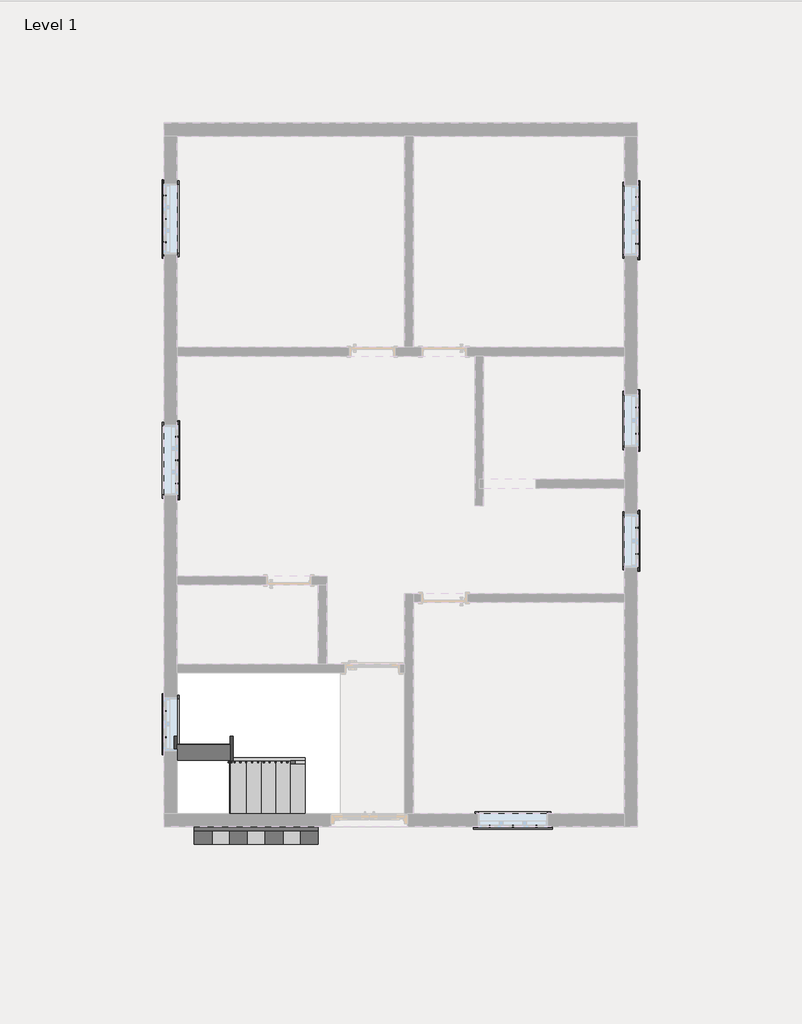
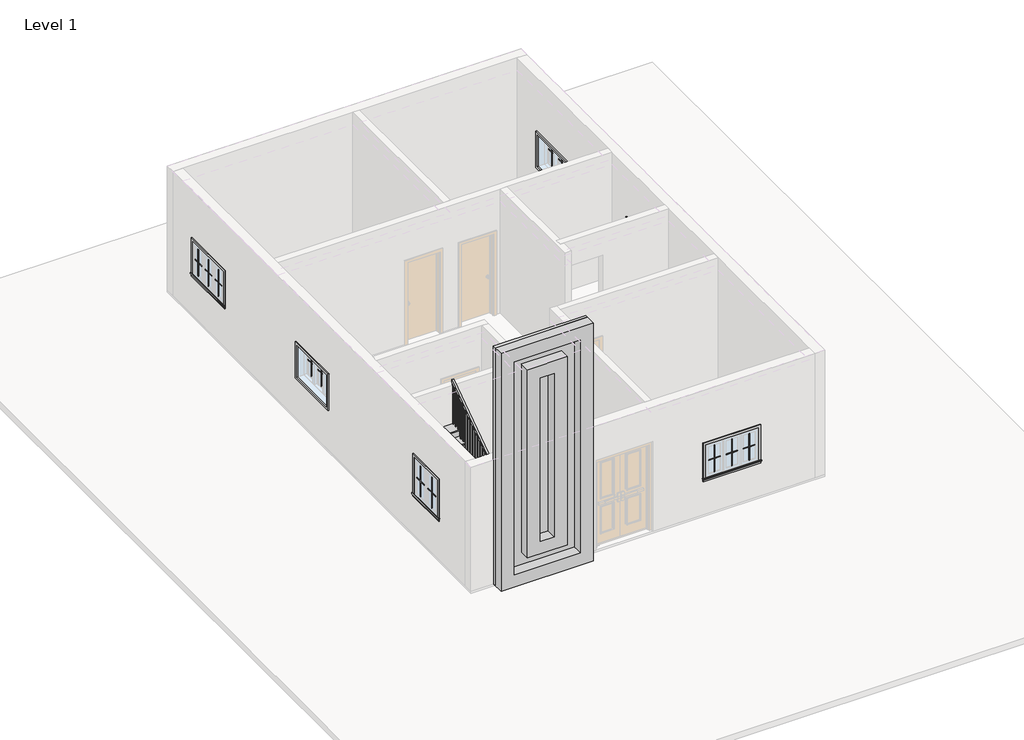
# One storey, part 2 of 2: 33 proxies, 6 members, 2 stair flights, 1 railing.
"""IFC4 building model written with IfcOpenShell, lengths in millimetres."""

from ifc_helpers import new_model, si_unit, frame, origin, place, context, project, spatial, polyline, outline, extrude, faceted_brep, transform, mapped, element, save
from components import design_design_9549e9b3, m_muntin_pattern_2x2_m_muntin_pattern_2x2_777d393c, m_muntin_pattern_2x2_m_muntin_pattern_2x2_fa3d06ac, m_muntin_pattern_2x2_m_muntin_pattern_2x2_55460d9e, m_muntin_pattern_2x2_m_muntin_pattern_2x2_a9b7b7a9, m_trim_window_exterior_flat_with_sill_3a557199, m_trim_window_exterior_flat_with_sill_8fa486dc, m_trim_window_interior_flat_picture_frame_580345df, m_trim_window_interior_flat_picture_frame_b6dd03a6, stair_flight_0f448409, stair_flight_de56df94

model = new_model("IFC4")

# Units and contexts
model_context = context("Model", 3, world=origin())
ifc_project = project(units=[si_unit("LENGTHUNIT", "METRE", prefix="MILLI")], contexts=[model_context])

# Site, building, storey
site = spatial("IfcSite", under=ifc_project)
building = spatial("IfcBuilding", under=site)
storey = spatial("IfcBuildingStorey", under=building, Name="Level 1", Elevation=0.0)

# Proxies
placement = place(None, origin())
design_design_shape = design_design_9549e9b3(model_context)
element("IfcBuildingElementProxy", 1, Name="DESIGN : DESIGN", ObjectType="DESIGN : DESIGN", at=placement, inside=storey, context=model_context, shape_type="MappedRepresentation", body=[
    mapped(design_design_shape, transform((0.0, 0.0, 0.0), x_axis=(1.0, 0.0, 0.0), y_axis=(0.0, 1.0, 0.0), z_axis=(0.0, 0.0, 1.0))),
])
m_muntin_pattern_2x2_m_muntin_pattern_2x2_shape = m_muntin_pattern_2x2_m_muntin_pattern_2x2_777d393c(model_context)
element("IfcBuildingElementProxy", 2, Name="M_Muntin Pattern_2x2 : M_Muntin Pattern_2x2", ObjectType="M_Muntin Pattern_2x2 : M_Muntin Pattern_2x2", at=placement, inside=storey, context=model_context, shape_type="MappedRepresentation", body=[
    mapped(m_muntin_pattern_2x2_m_muntin_pattern_2x2_shape, transform((-5759.4629317, 4113.1478103, 1111.25), x_axis=(0.0, 1.0, 0.0), y_axis=(-1.0, 0.0, 0.0), z_axis=(0.0, 0.0, 1.0))),
])
element("IfcBuildingElementProxy", 3, Name="M_Muntin Pattern_2x2 : M_Muntin Pattern_2x2", ObjectType="M_Muntin Pattern_2x2 : M_Muntin Pattern_2x2", at=placement, inside=storey, context=model_context, shape_type="MappedRepresentation", body=[
    mapped(m_muntin_pattern_2x2_m_muntin_pattern_2x2_shape, transform((2425.6870683, 4896.314477, 969.85), x_axis=(0.0, -1.0, 0.0), y_axis=(1.0, 0.0, 0.0), z_axis=(0.0, 0.0, 1.0))),
])
element("IfcBuildingElementProxy", 4, Name="M_Muntin Pattern_2x2 : M_Muntin Pattern_2x2", ObjectType="M_Muntin Pattern_2x2 : M_Muntin Pattern_2x2", at=placement, inside=storey, context=model_context, shape_type="MappedRepresentation", body=[
    mapped(m_muntin_pattern_2x2_m_muntin_pattern_2x2_shape, transform((-5549.9129317, 743.414477, 1111.25), x_axis=(0.0, -1.0, 0.0), y_axis=(1.0, 0.0, 0.0), z_axis=(0.0, 0.0, 1.0))),
])
element("IfcBuildingElementProxy", 5, Name="M_Muntin Pattern_2x2 : M_Muntin Pattern_2x2", ObjectType="M_Muntin Pattern_2x2 : M_Muntin Pattern_2x2", at=placement, inside=storey, context=model_context, shape_type="MappedRepresentation", body=[
    mapped(m_muntin_pattern_2x2_m_muntin_pattern_2x2_shape, transform((680.4954017, -6001.3438563, 969.85), x_axis=(-1.0, 0.0, 0.0), y_axis=(0.0, -1.0, 0.0), z_axis=(0.0, 0.0, 1.0))),
])
m_muntin_pattern_2x2_m_muntin_pattern_2x2_2_shape = m_muntin_pattern_2x2_m_muntin_pattern_2x2_fa3d06ac(model_context)
element("IfcBuildingElementProxy", 6, Name="M_Muntin Pattern_2x2 : M_Muntin Pattern_2x2", ObjectType="M_Muntin Pattern_2x2 : M_Muntin Pattern_2x2", at=placement, inside=storey, context=model_context, shape_type="MappedRepresentation", body=[
    mapped(m_muntin_pattern_2x2_m_muntin_pattern_2x2_2_shape, transform((-5759.4629317, 4921.714477, 1111.25), x_axis=(0.0, -1.0, 0.0), y_axis=(1.0, 0.0, 0.0), z_axis=(0.0, 0.0, 1.0))),
])
element("IfcBuildingElementProxy", 7, Name="M_Muntin Pattern_2x2 : M_Muntin Pattern_2x2", ObjectType="M_Muntin Pattern_2x2 : M_Muntin Pattern_2x2", at=placement, inside=storey, context=model_context, shape_type="MappedRepresentation", body=[
    mapped(m_muntin_pattern_2x2_m_muntin_pattern_2x2_2_shape, transform((-5759.4629317, 4517.4311437, 1111.25), x_axis=(0.0, -1.0, 0.0), y_axis=(1.0, 0.0, 0.0), z_axis=(0.0, 0.0, 1.0))),
])
element("IfcBuildingElementProxy", 8, Name="M_Muntin Pattern_2x2 : M_Muntin Pattern_2x2", ObjectType="M_Muntin Pattern_2x2 : M_Muntin Pattern_2x2", at=placement, inside=storey, context=model_context, shape_type="MappedRepresentation", body=[
    mapped(m_muntin_pattern_2x2_m_muntin_pattern_2x2_2_shape, transform((2425.6870683, 4087.7478103, 969.85), x_axis=(0.0, 1.0, 0.0), y_axis=(-1.0, 0.0, 0.0), z_axis=(0.0, 0.0, 1.0))),
])
element("IfcBuildingElementProxy", 9, Name="M_Muntin Pattern_2x2 : M_Muntin Pattern_2x2", ObjectType="M_Muntin Pattern_2x2 : M_Muntin Pattern_2x2", at=placement, inside=storey, context=model_context, shape_type="MappedRepresentation", body=[
    mapped(m_muntin_pattern_2x2_m_muntin_pattern_2x2_2_shape, transform((2425.6870683, 4492.0311437, 969.85), x_axis=(0.0, 1.0, 0.0), y_axis=(-1.0, 0.0, 0.0), z_axis=(0.0, 0.0, 1.0))),
])
element("IfcBuildingElementProxy", 10, Name="M_Muntin Pattern_2x2 : M_Muntin Pattern_2x2", ObjectType="M_Muntin Pattern_2x2 : M_Muntin Pattern_2x2", at=placement, inside=storey, context=model_context, shape_type="MappedRepresentation", body=[
    mapped(m_muntin_pattern_2x2_m_muntin_pattern_2x2_2_shape, transform((-5549.9129317, -65.1521897, 1111.25), x_axis=(0.0, 1.0, 0.0), y_axis=(-1.0, 0.0, 0.0), z_axis=(0.0, 0.0, 1.0))),
])
element("IfcBuildingElementProxy", 11, Name="M_Muntin Pattern_2x2 : M_Muntin Pattern_2x2", ObjectType="M_Muntin Pattern_2x2 : M_Muntin Pattern_2x2", at=placement, inside=storey, context=model_context, shape_type="MappedRepresentation", body=[
    mapped(m_muntin_pattern_2x2_m_muntin_pattern_2x2_2_shape, transform((-5549.9129317, 339.1311437, 1111.25), x_axis=(0.0, 1.0, 0.0), y_axis=(-1.0, 0.0, 0.0), z_axis=(0.0, 0.0, 1.0))),
])
element("IfcBuildingElementProxy", 12, Name="M_Muntin Pattern_2x2 : M_Muntin Pattern_2x2", ObjectType="M_Muntin Pattern_2x2 : M_Muntin Pattern_2x2", at=placement, inside=storey, context=model_context, shape_type="MappedRepresentation", body=[
    mapped(m_muntin_pattern_2x2_m_muntin_pattern_2x2_2_shape, transform((-128.071265, -6001.3438563, 969.85), x_axis=(1.0, 0.0, 0.0), y_axis=(0.0, 1.0, 0.0), z_axis=(0.0, 0.0, 1.0))),
])
element("IfcBuildingElementProxy", 13, Name="M_Muntin Pattern_2x2 : M_Muntin Pattern_2x2", ObjectType="M_Muntin Pattern_2x2 : M_Muntin Pattern_2x2", at=placement, inside=storey, context=model_context, shape_type="MappedRepresentation", body=[
    mapped(m_muntin_pattern_2x2_m_muntin_pattern_2x2_2_shape, transform((276.2120683, -6001.3438563, 969.85), x_axis=(1.0, 0.0, 0.0), y_axis=(0.0, 1.0, 0.0), z_axis=(0.0, 0.0, 1.0))),
])
m_muntin_pattern_2x2_m_muntin_pattern_2x2_3_shape = m_muntin_pattern_2x2_m_muntin_pattern_2x2_55460d9e(model_context)
element("IfcBuildingElementProxy", 14, Name="M_Muntin Pattern_2x2 : M_Muntin Pattern_2x2", ObjectType="M_Muntin Pattern_2x2 : M_Muntin Pattern_2x2", at=placement, inside=storey, context=model_context, shape_type="MappedRepresentation", body=[
    mapped(m_muntin_pattern_2x2_m_muntin_pattern_2x2_3_shape, transform((-5759.4629317, -4459.8813563, 1111.25), x_axis=(0.0, 1.0, 0.0), y_axis=(-1.0, 0.0, 0.0), z_axis=(0.0, 0.0, 1.0))),
])
element("IfcBuildingElementProxy", 15, Name="M_Muntin Pattern_2x2 : M_Muntin Pattern_2x2", ObjectType="M_Muntin Pattern_2x2 : M_Muntin Pattern_2x2", at=placement, inside=storey, context=model_context, shape_type="MappedRepresentation", body=[
    mapped(m_muntin_pattern_2x2_m_muntin_pattern_2x2_3_shape, transform((2425.6870683, -830.8563563, 969.85), x_axis=(0.0, -1.0, 0.0), y_axis=(1.0, 0.0, 0.0), z_axis=(0.0, 0.0, 1.0))),
])
element("IfcBuildingElementProxy", 16, Name="M_Muntin Pattern_2x2 : M_Muntin Pattern_2x2", ObjectType="M_Muntin Pattern_2x2 : M_Muntin Pattern_2x2", at=placement, inside=storey, context=model_context, shape_type="MappedRepresentation", body=[
    mapped(m_muntin_pattern_2x2_m_muntin_pattern_2x2_3_shape, transform((2425.6870683, 1251.9436437, 969.85), x_axis=(0.0, -1.0, 0.0), y_axis=(1.0, 0.0, 0.0), z_axis=(0.0, 0.0, 1.0))),
])
m_muntin_pattern_2x2_m_muntin_pattern_2x2_4_shape = m_muntin_pattern_2x2_m_muntin_pattern_2x2_a9b7b7a9(model_context)
element("IfcBuildingElementProxy", 17, Name="M_Muntin Pattern_2x2 : M_Muntin Pattern_2x2", ObjectType="M_Muntin Pattern_2x2 : M_Muntin Pattern_2x2", at=placement, inside=storey, context=model_context, shape_type="MappedRepresentation", body=[
    mapped(m_muntin_pattern_2x2_m_muntin_pattern_2x2_4_shape, transform((-5759.4629317, -4005.8563563, 1111.25), x_axis=(0.0, -1.0, 0.0), y_axis=(1.0, 0.0, 0.0), z_axis=(0.0, 0.0, 1.0))),
])
element("IfcBuildingElementProxy", 18, Name="M_Muntin Pattern_2x2 : M_Muntin Pattern_2x2", ObjectType="M_Muntin Pattern_2x2 : M_Muntin Pattern_2x2", at=placement, inside=storey, context=model_context, shape_type="MappedRepresentation", body=[
    mapped(m_muntin_pattern_2x2_m_muntin_pattern_2x2_4_shape, transform((2425.6870683, -1284.8813563, 969.85), x_axis=(0.0, 1.0, 0.0), y_axis=(-1.0, 0.0, 0.0), z_axis=(0.0, 0.0, 1.0))),
])
element("IfcBuildingElementProxy", 19, Name="M_Muntin Pattern_2x2 : M_Muntin Pattern_2x2", ObjectType="M_Muntin Pattern_2x2 : M_Muntin Pattern_2x2", at=placement, inside=storey, context=model_context, shape_type="MappedRepresentation", body=[
    mapped(m_muntin_pattern_2x2_m_muntin_pattern_2x2_4_shape, transform((2425.6870683, 797.9186437, 969.85), x_axis=(0.0, 1.0, 0.0), y_axis=(-1.0, 0.0, 0.0), z_axis=(0.0, 0.0, 1.0))),
])
m_trim_window_exterior_flat_with_sill_shape = m_trim_window_exterior_flat_with_sill_3a557199(model_context)
element("IfcBuildingElementProxy", 20, Name="M_Trim-Window-Exterior-Flat : with Sill", ObjectType="M_Trim-Window-Exterior-Flat : with Sill", at=placement, inside=storey, context=model_context, shape_type="MappedRepresentation", body=[
    mapped(m_trim_window_exterior_flat_with_sill_shape, transform((-5768.9879317, 4517.4311437, 1841.4), x_axis=(0.0, -1.0, 0.0), y_axis=(0.0, 0.0, 1.0), z_axis=(-1.0, 0.0, 0.0))),
])
element("IfcBuildingElementProxy", 21, Name="M_Trim-Window-Exterior-Flat : with Sill", ObjectType="M_Trim-Window-Exterior-Flat : with Sill", at=placement, inside=storey, context=model_context, shape_type="MappedRepresentation", body=[
    mapped(m_trim_window_exterior_flat_with_sill_shape, transform((2435.2120683, 4492.0311437, 1700.0), x_axis=(0.0, 1.0, 0.0), y_axis=(0.0, 0.0, 1.0), z_axis=(1.0, 0.0, 0.0))),
])
element("IfcBuildingElementProxy", 22, Name="M_Trim-Window-Exterior-Flat : with Sill", ObjectType="M_Trim-Window-Exterior-Flat : with Sill", at=placement, inside=storey, context=model_context, shape_type="MappedRepresentation", body=[
    mapped(m_trim_window_exterior_flat_with_sill_shape, transform((-5540.3879317, 339.1311437, 1841.4), x_axis=(0.0, 1.0, 0.0), y_axis=(0.0, 0.0, 1.0), z_axis=(1.0, 0.0, 0.0))),
])
element("IfcBuildingElementProxy", 23, Name="M_Trim-Window-Exterior-Flat : with Sill", ObjectType="M_Trim-Window-Exterior-Flat : with Sill", at=placement, inside=storey, context=model_context, shape_type="MappedRepresentation", body=[
    mapped(m_trim_window_exterior_flat_with_sill_shape, transform((276.2120683, -6010.8688563, 1700.0), x_axis=(1.0, 0.0, 0.0), y_axis=(0.0, 0.0, 1.0), z_axis=(0.0, -1.0, 0.0))),
])
m_trim_window_exterior_flat_with_sill_2_shape = m_trim_window_exterior_flat_with_sill_8fa486dc(model_context)
element("IfcBuildingElementProxy", 24, Name="M_Trim-Window-Exterior-Flat : with Sill", ObjectType="M_Trim-Window-Exterior-Flat : with Sill", at=placement, inside=storey, context=model_context, shape_type="MappedRepresentation", body=[
    mapped(m_trim_window_exterior_flat_with_sill_2_shape, transform((-5768.9879317, -4232.8688563, 1941.4), x_axis=(0.0, -1.0, 0.0), y_axis=(0.0, 0.0, 1.0), z_axis=(-1.0, 0.0, 0.0))),
])
element("IfcBuildingElementProxy", 25, Name="M_Trim-Window-Exterior-Flat : with Sill", ObjectType="M_Trim-Window-Exterior-Flat : with Sill", at=placement, inside=storey, context=model_context, shape_type="MappedRepresentation", body=[
    mapped(m_trim_window_exterior_flat_with_sill_2_shape, transform((2435.2120683, -1057.8688563, 1800.0), x_axis=(0.0, 1.0, 0.0), y_axis=(0.0, 0.0, 1.0), z_axis=(1.0, 0.0, 0.0))),
])
element("IfcBuildingElementProxy", 26, Name="M_Trim-Window-Exterior-Flat : with Sill", ObjectType="M_Trim-Window-Exterior-Flat : with Sill", at=placement, inside=storey, context=model_context, shape_type="MappedRepresentation", body=[
    mapped(m_trim_window_exterior_flat_with_sill_2_shape, transform((2435.2120683, 1024.9311437, 1800.0), x_axis=(0.0, 1.0, 0.0), y_axis=(0.0, 0.0, 1.0), z_axis=(1.0, 0.0, 0.0))),
])
m_trim_window_interior_flat_picture_frame_shape = m_trim_window_interior_flat_picture_frame_580345df(model_context)
element("IfcBuildingElementProxy", 27, Name="M_Trim-Window-Interior-Flat : Picture Frame", ObjectType="M_Trim-Window-Interior-Flat : Picture Frame", at=placement, inside=storey, context=model_context, shape_type="MappedRepresentation", body=[
    mapped(m_trim_window_interior_flat_picture_frame_shape, transform((-5540.3879317, 4517.4311437, 1841.4), x_axis=(0.0, 1.0, 0.0), y_axis=(0.0, 0.0, 1.0), z_axis=(1.0, 0.0, 0.0))),
])
element("IfcBuildingElementProxy", 28, Name="M_Trim-Window-Interior-Flat : Picture Frame", ObjectType="M_Trim-Window-Interior-Flat : Picture Frame", at=placement, inside=storey, context=model_context, shape_type="MappedRepresentation", body=[
    mapped(m_trim_window_interior_flat_picture_frame_shape, transform((2206.6120683, 4492.0311437, 1700.0), x_axis=(0.0, -1.0, 0.0), y_axis=(0.0, 0.0, 1.0), z_axis=(-1.0, 0.0, 0.0))),
])
element("IfcBuildingElementProxy", 29, Name="M_Trim-Window-Interior-Flat : Picture Frame", ObjectType="M_Trim-Window-Interior-Flat : Picture Frame", at=placement, inside=storey, context=model_context, shape_type="MappedRepresentation", body=[
    mapped(m_trim_window_interior_flat_picture_frame_shape, transform((-5768.9879317, 339.1311437, 1841.4), x_axis=(0.0, -1.0, 0.0), y_axis=(0.0, 0.0, 1.0), z_axis=(-1.0, 0.0, 0.0))),
])
element("IfcBuildingElementProxy", 30, Name="M_Trim-Window-Interior-Flat : Picture Frame", ObjectType="M_Trim-Window-Interior-Flat : Picture Frame", at=placement, inside=storey, context=model_context, shape_type="MappedRepresentation", body=[
    mapped(m_trim_window_interior_flat_picture_frame_shape, transform((276.2120683, -5782.2688563, 1700.0), x_axis=(-1.0, 0.0, 0.0), y_axis=(0.0, 0.0, 1.0), z_axis=(0.0, 1.0, 0.0))),
])
m_trim_window_interior_flat_picture_frame_2_shape = m_trim_window_interior_flat_picture_frame_b6dd03a6(model_context)
element("IfcBuildingElementProxy", 31, Name="M_Trim-Window-Interior-Flat : Picture Frame", ObjectType="M_Trim-Window-Interior-Flat : Picture Frame", at=placement, inside=storey, context=model_context, shape_type="MappedRepresentation", body=[
    mapped(m_trim_window_interior_flat_picture_frame_2_shape, transform((-5540.3879317, -4232.8688563, 1941.4), x_axis=(0.0, 1.0, 0.0), y_axis=(0.0, 0.0, 1.0), z_axis=(1.0, 0.0, 0.0))),
])
element("IfcBuildingElementProxy", 32, Name="M_Trim-Window-Interior-Flat : Picture Frame", ObjectType="M_Trim-Window-Interior-Flat : Picture Frame", at=placement, inside=storey, context=model_context, shape_type="MappedRepresentation", body=[
    mapped(m_trim_window_interior_flat_picture_frame_2_shape, transform((2206.6120683, -1057.8688563, 1800.0), x_axis=(0.0, -1.0, 0.0), y_axis=(0.0, 0.0, 1.0), z_axis=(-1.0, 0.0, 0.0))),
])
element("IfcBuildingElementProxy", 33, Name="M_Trim-Window-Interior-Flat : Picture Frame", ObjectType="M_Trim-Window-Interior-Flat : Picture Frame", at=placement, inside=storey, context=model_context, shape_type="MappedRepresentation", body=[
    mapped(m_trim_window_interior_flat_picture_frame_2_shape, transform((2206.6120683, 1024.9311437, 1800.0), x_axis=(0.0, -1.0, 0.0), y_axis=(0.0, 0.0, 1.0), z_axis=(-1.0, 0.0, 0.0))),
])

# Members
element("IfcMember", 34, ObjectType="Stringer - 2\" Width", at=placement, inside=storey, context=model_context, shape_type="SweptSolid", body=[
    extrude(outline(polyline([(0.0, -3329.9669727), (220.7029228, -3329.9669727), (1131.2769231, -4645.2405286), (826.4769231, -4740.452879), (0.0, -3546.652879), (0.0, -3329.9669727)])), frame((0.0, -5833.0688563, 0.0), z_axis=(0.0, 1.0, 0.0), x_axis=(0.0, 0.0, 1.0)), (0.0, 0.0, 1.0), 50.8),
])
element("IfcMember", 35, ObjectType="Stringer - 2\" Width", at=placement, inside=storey, context=model_context, shape_type="SweptSolid", body=[
    extrude(outline(polyline([(0.0, -3329.9669727), (220.7029228, -3329.9669727), (1082.7789714, -4575.1879317), (712.0627288, -4575.1879317), (0.0, -3546.652879), (0.0, -3329.9669727)])), frame((0.0, -4867.8688563, 0.0), z_axis=(0.0, 1.0, 0.0), x_axis=(0.0, 0.0, 1.0)), (0.0, 0.0, 1.0), 50.8),
])
element("IfcMember", 36, ObjectType="Stringer - 2\" Width", at=placement, inside=storey, context=model_context, shape_type="SweptSolid", body=[
    extrude(outline(polyline([(-4981.38295, 826.4769231), (-5076.5953004, 1131.2769231), (-3343.8688563, 2330.856769), (-3343.8688563, 1960.1405264), (-4981.38295, 826.4769231)])), frame((-5591.1879317, 0.0, 0.0), z_axis=(1.0, 0.0, 0.0), x_axis=(0.0, 1.0, 0.0)), (0.0, 0.0, 1.0), 50.8),
])
element("IfcMember", 37, ObjectType="Stringer - 2\" Width", at=placement, inside=storey, context=model_context, shape_type="SweptSolid", body=[
    extrude(outline(polyline([(-4867.8688563, 905.0636033), (-4867.8688563, 1275.7798459), (-3343.8688563, 2330.856769), (-3343.8688563, 1960.1405264), (-4867.8688563, 905.0636033)])), frame((-4625.9879317, 0.0, 0.0), z_axis=(1.0, 0.0, 0.0), x_axis=(0.0, 1.0, 0.0)), (0.0, 0.0, 1.0), 50.8),
])
element("IfcMember", 38, ObjectType="Stringer - 2\" Width", at=placement, inside=storey, context=model_context, shape_type="Brep", body=[
    faceted_brep([(-5540.3879317, -5076.5953004, 1131.2769231), (-5591.1879317, -5076.5953004, 1131.2769231), (-5591.1879317, -5833.0688563, 1131.2769231), (-5540.3879317, -5782.2688563, 1131.2769231), (-5540.3879317, -4981.38295, 826.4769231), (-5540.3879317, -5782.2688563, 826.4769231), (-5591.1879317, -4981.38295, 826.4769231), (-5591.1879317, -5833.0688563, 826.4769231)], [[[0, 1, 2, 3]], [[4, 0, 3, 5]], [[6, 4, 5, 7]], [[1, 6, 7, 2]], [[1, 0, 4, 6]], [[2, 7, 5, 3]]]),
])
element("IfcMember", 39, ObjectType="Stringer - 2\" Width", at=placement, inside=storey, context=model_context, shape_type="Brep", body=[
    faceted_brep([(-5540.3879317, -5782.2688563, 1131.2769231), (-5591.1879317, -5833.0688563, 1131.2769231), (-4645.2405286, -5833.0688563, 1131.2769231), (-4645.2405286, -5782.2688563, 1131.2769231), (-5540.3879317, -5782.2688563, 826.4769231), (-4740.452879, -5782.2688563, 826.4769231), (-5591.1879317, -5833.0688563, 826.4769231), (-4740.452879, -5833.0688563, 826.4769231)], [[[0, 1, 2, 3]], [[4, 0, 3, 5]], [[6, 4, 5, 7]], [[1, 6, 7, 2]], [[1, 0, 4, 6]], [[2, 7, 5, 3]]]),
])

# Railing
element("IfcRailing", 40, ObjectType="Handrail - Rectangular", at=placement, inside=storey, context=model_context, shape_type="SolidModel", body=[
    faceted_brep([(-3329.9669727, -4918.6688563, 1090.2461538), (-3329.9669727, -4918.6688563, 1028.4601134), (-3329.9669727, -4867.8688563, 1028.4601134), (-3329.9669727, -4867.8688563, 1090.2461538), (-4599.9669727, -4918.6688563, 1969.4769231), (-4615.8356977, -4918.6688563, 1918.6769231), (-4615.8356977, -4867.8688563, 1918.6769231), (-4599.9669727, -4867.8688563, 1969.4769231), (-4625.9879317, -4918.6688563, 1969.4769231), (-4625.9879317, -4867.8688563, 1969.4769231), (-4676.7879317, -4867.8688563, 1918.6769231), (-4676.7879317, -4918.6688563, 1918.6769231)], [[[0, 1, 2, 3]], [[1, 0, 4, 5]], [[2, 1, 5, 6]], [[3, 2, 6, 7]], [[0, 3, 7, 4]], [[8, 9, 10, 11]], [[5, 4, 8, 11]], [[6, 5, 11, 10]], [[7, 6, 10, 9]], [[4, 7, 9, 8]]]),
    faceted_brep([(-4625.9879317, -4918.6688563, 1969.4769231), (-4676.7879317, -4918.6688563, 1918.6769231), (-4676.7879317, -4867.8688563, 1918.6769231), (-4625.9879317, -4867.8688563, 1969.4769231), (-4625.9879317, -4918.6688563, 2110.1538462), (-4625.9879317, -4867.8688563, 2083.5370365), (-4676.7879317, -4867.8688563, 2083.5370365), (-4676.7879317, -4918.6688563, 2110.1538462)], [[[0, 1, 2, 3]], [[4, 5, 6, 7]], [[1, 0, 4, 7]], [[2, 1, 7, 6]], [[3, 2, 6, 5]], [[0, 3, 5, 4]]]),
    faceted_brep([(-4676.7879317, -4918.6688563, 2110.1538462), (-4676.7879317, -4867.8688563, 2083.5370365), (-4625.9879317, -4867.8688563, 2083.5370365), (-4625.9879317, -4918.6688563, 2110.1538462), (-4676.7879317, -3343.8688563, 3200.4), (-4625.9879317, -3343.8688563, 3200.4), (-4625.9879317, -3343.8688563, 3138.6139596), (-4676.7879317, -3343.8688563, 3138.6139596)], [[[0, 1, 2, 3]], [[4, 5, 6, 7]], [[1, 0, 4, 7]], [[2, 1, 7, 6]], [[3, 2, 6, 5]], [[0, 3, 5, 4]]]),
    extrude(outline(polyline([(-3378.7938563, 3114.4351134), (-3359.7438563, 3127.6235749), (-3359.7438563, 2110.1538462), (-3378.7938563, 2110.1538462), (-3378.7938563, 3114.4351134)])), frame((-4660.9129317, 0.0, 0.0), z_axis=(1.0, 0.0, 0.0), x_axis=(0.0, 1.0, 0.0)), (0.0, 0.0, 1.0), 19.05),
    extrude(outline(polyline([(-3480.3938563, 3044.0966519), (-3461.3438563, 3057.2851134), (-3461.3438563, 2110.1538462), (-3480.3938563, 2110.1538462), (-3480.3938563, 3044.0966519)])), frame((-4660.9129317, 0.0, 0.0), z_axis=(1.0, 0.0, 0.0), x_axis=(0.0, 1.0, 0.0)), (0.0, 0.0, 1.0), 19.05),
    extrude(outline(polyline([(-3581.9938563, 2973.7581903), (-3562.9438563, 2986.9466519), (-3562.9438563, 2110.1538462), (-3581.9938563, 2110.1538462), (-3581.9938563, 2973.7581903)])), frame((-4660.9129317, 0.0, 0.0), z_axis=(1.0, 0.0, 0.0), x_axis=(0.0, 1.0, 0.0)), (0.0, 0.0, 1.0), 19.05),
    extrude(outline(polyline([(-3683.5938563, 2903.4197288), (-3664.5438563, 2916.6081903), (-3664.5438563, 1934.3076923), (-3683.5938563, 1934.3076923), (-3683.5938563, 2903.4197288)])), frame((-4660.9129317, 0.0, 0.0), z_axis=(1.0, 0.0, 0.0), x_axis=(0.0, 1.0, 0.0)), (0.0, 0.0, 1.0), 19.05),
    extrude(outline(polyline([(-3785.1938563, 2833.0812673), (-3766.1438563, 2846.2697288), (-3766.1438563, 1934.3076923), (-3785.1938563, 1934.3076923), (-3785.1938563, 2833.0812673)])), frame((-4660.9129317, 0.0, 0.0), z_axis=(1.0, 0.0, 0.0), x_axis=(0.0, 1.0, 0.0)), (0.0, 0.0, 1.0), 19.05),
    extrude(outline(polyline([(-3886.7938563, 2762.7428057), (-3867.7438563, 2775.9312673), (-3867.7438563, 1758.4615385), (-3886.7938563, 1758.4615385), (-3886.7938563, 2762.7428057)])), frame((-4660.9129317, 0.0, 0.0), z_axis=(1.0, 0.0, 0.0), x_axis=(0.0, 1.0, 0.0)), (0.0, 0.0, 1.0), 19.05),
    extrude(outline(polyline([(-3988.3938563, 2692.4043442), (-3969.3438563, 2705.5928057), (-3969.3438563, 1758.4615385), (-3988.3938563, 1758.4615385), (-3988.3938563, 2692.4043442)])), frame((-4660.9129317, 0.0, 0.0), z_axis=(1.0, 0.0, 0.0), x_axis=(0.0, 1.0, 0.0)), (0.0, 0.0, 1.0), 19.05),
    extrude(outline(polyline([(-4089.9938563, 2622.0658826), (-4070.9438563, 2635.2543442), (-4070.9438563, 1758.4615385), (-4089.9938563, 1758.4615385), (-4089.9938563, 2622.0658826)])), frame((-4660.9129317, 0.0, 0.0), z_axis=(1.0, 0.0, 0.0), x_axis=(0.0, 1.0, 0.0)), (0.0, 0.0, 1.0), 19.05),
    extrude(outline(polyline([(-4191.5938563, 2551.7274211), (-4172.5438563, 2564.9158826), (-4172.5438563, 1582.6153846), (-4191.5938563, 1582.6153846), (-4191.5938563, 2551.7274211)])), frame((-4660.9129317, 0.0, 0.0), z_axis=(1.0, 0.0, 0.0), x_axis=(0.0, 1.0, 0.0)), (0.0, 0.0, 1.0), 19.05),
    extrude(outline(polyline([(-4293.1938563, 2481.3889596), (-4274.1438563, 2494.5774211), (-4274.1438563, 1582.6153846), (-4293.1938563, 1582.6153846), (-4293.1938563, 2481.3889596)])), frame((-4660.9129317, 0.0, 0.0), z_axis=(1.0, 0.0, 0.0), x_axis=(0.0, 1.0, 0.0)), (0.0, 0.0, 1.0), 19.05),
    extrude(outline(polyline([(-4394.7938563, 2411.050498), (-4375.7438563, 2424.2389596), (-4375.7438563, 1406.7692308), (-4394.7938563, 1406.7692308), (-4394.7938563, 2411.050498)])), frame((-4660.9129317, 0.0, 0.0), z_axis=(1.0, 0.0, 0.0), x_axis=(0.0, 1.0, 0.0)), (0.0, 0.0, 1.0), 19.05),
    extrude(outline(polyline([(-4496.3938563, 2340.7120365), (-4477.3438563, 2353.900498), (-4477.3438563, 1406.7692308), (-4496.3938563, 1406.7692308), (-4496.3938563, 2340.7120365)])), frame((-4660.9129317, 0.0, 0.0), z_axis=(1.0, 0.0, 0.0), x_axis=(0.0, 1.0, 0.0)), (0.0, 0.0, 1.0), 19.05),
    extrude(outline(polyline([(-4597.9938563, 2270.3735749), (-4578.9438563, 2283.5620365), (-4578.9438563, 1406.7692308), (-4597.9938563, 1406.7692308), (-4597.9938563, 2270.3735749)])), frame((-4660.9129317, 0.0, 0.0), z_axis=(1.0, 0.0, 0.0), x_axis=(0.0, 1.0, 0.0)), (0.0, 0.0, 1.0), 19.05),
    extrude(outline(polyline([(-4699.5938563, 2200.0351134), (-4680.5438563, 2213.2235749), (-4680.5438563, 1230.9230769), (-4699.5938563, 1230.9230769), (-4699.5938563, 2200.0351134)])), frame((-4660.9129317, 0.0, 0.0), z_axis=(1.0, 0.0, 0.0), x_axis=(0.0, 1.0, 0.0)), (0.0, 0.0, 1.0), 19.05),
    extrude(outline(polyline([(-4801.1938563, 2129.6966519), (-4782.1438563, 2142.8851134), (-4782.1438563, 1230.9230769), (-4801.1938563, 1230.9230769), (-4801.1938563, 2129.6966519)])), frame((-4660.9129317, 0.0, 0.0), z_axis=(1.0, 0.0, 0.0), x_axis=(0.0, 1.0, 0.0)), (0.0, 0.0, 1.0), 19.05),
    extrude(outline(polyline([(1865.9274211, -4539.6419727), (1879.1158826, -4558.6919727), (879.2307692, -4558.6919727), (879.2307692, -4539.6419727), (1865.9274211, -4539.6419727)])), frame((0.0, -4902.7938563, 0.0), z_axis=(0.0, 1.0, 0.0), x_axis=(0.0, 0.0, 1.0)), (0.0, 0.0, 1.0), 19.05),
    extrude(outline(polyline([(1795.5889596, -4438.0419727), (1808.7774211, -4457.0919727), (879.2307692, -4457.0919727), (879.2307692, -4438.0419727), (1795.5889596, -4438.0419727)])), frame((0.0, -4902.7938563, 0.0), z_axis=(0.0, 1.0, 0.0), x_axis=(0.0, 0.0, 1.0)), (0.0, 0.0, 1.0), 19.05),
    extrude(outline(polyline([(1725.250498, -4336.4419727), (1738.4389596, -4355.4919727), (879.2307692, -4355.4919727), (879.2307692, -4336.4419727), (1725.250498, -4336.4419727)])), frame((0.0, -4902.7938563, 0.0), z_axis=(0.0, 1.0, 0.0), x_axis=(0.0, 0.0, 1.0)), (0.0, 0.0, 1.0), 19.05),
    extrude(outline(polyline([(1654.9120365, -4234.8419727), (1668.100498, -4253.8919727), (703.3846154, -4253.8919727), (703.3846154, -4234.8419727), (1654.9120365, -4234.8419727)])), frame((0.0, -4902.7938563, 0.0), z_axis=(0.0, 1.0, 0.0), x_axis=(0.0, 0.0, 1.0)), (0.0, 0.0, 1.0), 19.05),
    extrude(outline(polyline([(1584.5735749, -4133.2419727), (1597.7620365, -4152.2919727), (703.3846154, -4152.2919727), (703.3846154, -4133.2419727), (1584.5735749, -4133.2419727)])), frame((0.0, -4902.7938563, 0.0), z_axis=(0.0, 1.0, 0.0), x_axis=(0.0, 0.0, 1.0)), (0.0, 0.0, 1.0), 19.05),
    extrude(outline(polyline([(1514.2351134, -4031.6419727), (1527.4235749, -4050.6919727), (527.5384615, -4050.6919727), (527.5384615, -4031.6419727), (1514.2351134, -4031.6419727)])), frame((0.0, -4902.7938563, 0.0), z_axis=(0.0, 1.0, 0.0), x_axis=(0.0, 0.0, 1.0)), (0.0, 0.0, 1.0), 19.05),
    extrude(outline(polyline([(1443.8966519, -3930.0419727), (1457.0851134, -3949.0919727), (527.5384615, -3949.0919727), (527.5384615, -3930.0419727), (1443.8966519, -3930.0419727)])), frame((0.0, -4902.7938563, 0.0), z_axis=(0.0, 1.0, 0.0), x_axis=(0.0, 0.0, 1.0)), (0.0, 0.0, 1.0), 19.05),
    extrude(outline(polyline([(1373.5581903, -3828.4419727), (1386.7466519, -3847.4919727), (527.5384615, -3847.4919727), (527.5384615, -3828.4419727), (1373.5581903, -3828.4419727)])), frame((0.0, -4902.7938563, 0.0), z_axis=(0.0, 1.0, 0.0), x_axis=(0.0, 0.0, 1.0)), (0.0, 0.0, 1.0), 19.05),
    extrude(outline(polyline([(1303.2197288, -3726.8419727), (1316.4081903, -3745.8919727), (351.6923077, -3745.8919727), (351.6923077, -3726.8419727), (1303.2197288, -3726.8419727)])), frame((0.0, -4902.7938563, 0.0), z_axis=(0.0, 1.0, 0.0), x_axis=(0.0, 0.0, 1.0)), (0.0, 0.0, 1.0), 19.05),
    extrude(outline(polyline([(1232.8812673, -3625.2419727), (1246.0697288, -3644.2919727), (351.6923077, -3644.2919727), (351.6923077, -3625.2419727), (1232.8812673, -3625.2419727)])), frame((0.0, -4902.7938563, 0.0), z_axis=(0.0, 1.0, 0.0), x_axis=(0.0, 0.0, 1.0)), (0.0, 0.0, 1.0), 19.05),
    extrude(outline(polyline([(1162.5428057, -3523.6419727), (1175.7312673, -3542.6919727), (175.8461538, -3542.6919727), (175.8461538, -3523.6419727), (1162.5428057, -3523.6419727)])), frame((0.0, -4902.7938563, 0.0), z_axis=(0.0, 1.0, 0.0), x_axis=(0.0, 0.0, 1.0)), (0.0, 0.0, 1.0), 19.05),
    extrude(outline(polyline([(1092.2043442, -3422.0419727), (1105.3928057, -3441.0919727), (175.8461538, -3441.0919727), (175.8461538, -3422.0419727), (1092.2043442, -3422.0419727)])), frame((0.0, -4902.7938563, 0.0), z_axis=(0.0, 1.0, 0.0), x_axis=(0.0, 0.0, 1.0)), (0.0, 0.0, 1.0), 19.05),
    extrude(outline(polyline([(-4641.8629317, -4883.7438563), (-4641.8629317, -4902.7938563), (-4660.9129317, -4902.7938563), (-4660.9129317, -4883.7438563), (-4641.8629317, -4883.7438563)])), frame((0.0, 0.0, 1055.0769231), z_axis=(0.0, 0.0, 1.0), x_axis=(1.0, 0.0, 0.0)), (0.0, 0.0, 1.0), 863.6),
    extrude(outline(polyline([(1901.0966519, -4590.4419727), (1914.2851134, -4609.4919727), (1055.0769231, -4609.4919727), (1055.0769231, -4590.4419727), (1901.0966519, -4590.4419727)])), frame((0.0, -4902.7938563, 0.0), z_axis=(0.0, 1.0, 0.0), x_axis=(0.0, 0.0, 1.0)), (0.0, 0.0, 1.0), 19.05),
    extrude(outline(polyline([(-3362.9188563, 3125.425498), (-3343.8688563, 3138.6139596), (-3343.8688563, 2110.1538462), (-3362.9188563, 2110.1538462), (-3362.9188563, 3125.425498)])), frame((-4660.9129317, 0.0, 0.0), z_axis=(1.0, 0.0, 0.0), x_axis=(0.0, 1.0, 0.0)), (0.0, 0.0, 1.0), 19.05),
    extrude(outline(polyline([(1028.4601134, -3329.9669727), (1041.6485749, -3349.0169727), (175.8461538, -3349.0169727), (175.8461538, -3329.9669727), (1028.4601134, -3329.9669727)])), frame((0.0, -4902.7938563, 0.0), z_axis=(0.0, 1.0, 0.0), x_axis=(0.0, 0.0, 1.0)), (0.0, 0.0, 1.0), 19.05),
])

# Stair flights
stair_flight_shape = stair_flight_0f448409(model_context)
element("IfcStairFlight", 41, ObjectType="2\" Tread 1\" Nosing 1/4\" Riser", at=placement, inside=storey, context=model_context, shape_type="MappedRepresentation", body=[
    mapped(stair_flight_shape, transform((0.0, 0.0, 0.0), x_axis=(1.0, 0.0, 0.0), y_axis=(0.0, 1.0, 0.0), z_axis=(0.0, 0.0, 1.0))),
])
stair_flight_2_shape = stair_flight_de56df94(model_context)
element("IfcStairFlight", 42, ObjectType="2\" Tread 1\" Nosing 1/4\" Riser", at=placement, inside=storey, context=model_context, shape_type="MappedRepresentation", body=[
    mapped(stair_flight_2_shape, transform((0.0, 0.0, 0.0), x_axis=(1.0, 0.0, 0.0), y_axis=(0.0, 1.0, 0.0), z_axis=(0.0, 0.0, 1.0))),
])

save(model, "model.ifc")

# Revit data of these elements
# Type "M_Muntin Pattern_2x2 : M_Muntin Pattern_2x2"
#   Width [instance default] = 3' - 11.24409"
#   Thickness = 0' - 0 1/2"
#   Height [instance default] = 3' - 11.24409"
#   Distance = 0' - 0 3/4"
#   Interior Material [instance default] = none
#   Exterior Material [instance default] = none
#   Default Elevation = 0
# Type "M_Trim-Window-Exterior-Flat : with Sill"
#   Trim Width = 0' - 2.3622"
#   Trim Thickness_Picture Frame = 0' - 1.1811"
#   Trim Thickness_with Sill = 0' - 0 3/4"
#   Sill Thickness = 0' - 1.1811"
#   Opening Width [instance default] = 1' - 11.62205"
#   Opening Height [instance default] = 2' - 11.43307"
#   Default Elevation = 3' - 11.24409"
#   Sill = yes
#   Picture Frame = no
#   Trim Material [instance default] = none
# Type "M_Trim-Window-Interior-Flat : Picture Frame"
#   Trim Thickness_Picture Frame = 0' - 1.1811"
#   Trim Width = 0' - 2.3622"
#   Trim Thickness_with Sill = 0' - 0.7874"
#   Sill Thickness = 0' - 1.1811"
#   Opening Width [instance default] = 1' - 11.62205"
#   Opening Height [instance default] = 2' - 11.43307"
#   Default Elevation = 3' - 11.24409"
#   Sill = no
#   Picture Frame = yes
#   Trim Material [instance default] = none
# Type "Handrail - Rectangular"
#   Assembly Code = "C2010400"
#   built-in parameter 1008612 = 0.0416667 (stored number, unit not read)
#   built-in parameter 1008611 = 0.0416667 (stored number, unit not read)
#   built-in parameter 1008609 = 0.333333 (stored number, unit not read)
#   built-in parameter 1008604 = 0.166667 (stored number, unit not read)
#   built-in parameter 1008603 = 0.166667 (stored number, unit not read)
#   Railing Height = 3' - 0"
#   built-in parameter 1008630 = 2
#   built-in parameter 1008610 = 2
#   built-in parameter 1008618 = Baluster - Square : 3/4"
# Element 1 (IfcBuildingElementProxy, "DESIGN : DESIGN")
#   Phase Created = New Construction
#   Materials on its faces: "PAINT 1", "Wood Planks"
# Elements 2, 3, 4, 5, 6, 7, 8, 9, 10, 11, 12, 13 (IfcBuildingElementProxy, "M_Muntin Pattern_2x2 : M_Muntin Pattern_2x2")
#   Width = 0' - 10.66667"
#   Height = 2' - 1.99606"
#   Interior Material = Wood - Stained
#   Exterior Material = Clad - White
#   Phase Created = New Construction
#   Materials on its faces: "Clad - White", "Wood - Stained"
# Elements 14, 15, 16, 17, 18, 19 (IfcBuildingElementProxy, "M_Muntin Pattern_2x2 : M_Muntin Pattern_2x2")
#   Width = 1' - 0 5/8"
#   Height = 2' - 5.93307"
#   Interior Material = Wood - Stained
#   Exterior Material = Clad - White
#   Phase Created = New Construction
#   Materials on its faces: "Clad - White", "Wood - Stained"
# Elements 20, 21, 22, 23 (IfcBuildingElementProxy, "M_Trim-Window-Exterior-Flat : with Sill")
#   Opening Width = 4' - 0"
#   Opening Height = 2' - 7.49606"
#   Trim Material = Clad - White
#   Phase Created = New Construction
#   Materials on its faces: "Clad - White"
# Elements 24, 25, 26 (IfcBuildingElementProxy, "M_Trim-Window-Exterior-Flat : with Sill")
#   Opening Width = 3' - 0"
#   Opening Height = 2' - 11.43307"
#   Trim Material = Clad - White
#   Phase Created = New Construction
#   Materials on its faces: "Clad - White"
# Elements 27, 28, 29, 30 (IfcBuildingElementProxy, "M_Trim-Window-Interior-Flat : Picture Frame")
#   Opening Width = 4' - 0"
#   Opening Height = 2' - 7.49606"
#   Trim Material = Wood - Stained
#   Phase Created = New Construction
#   Materials on its faces: "Wood - Stained"
# Elements 31, 32, 33 (IfcBuildingElementProxy, "M_Trim-Window-Interior-Flat : Picture Frame")
#   Opening Width = 3' - 0"
#   Opening Height = 2' - 11.43307"
#   Trim Material = Wood - Stained
#   Phase Created = New Construction
#   Materials on its faces: "Wood - Stained"
# Elements 34, 35, 36, 37, 38, 39 (IfcMember, "Stringer - 2\" Width")
#   Phase Created = New Construction
# Element 40 (IfcRailing, "Handrail - Rectangular")
#   Phase Created = New Construction
# Elements 41, 42 (IfcStairFlight, "2\" Tread 1\" Nosing 1/4\" Riser")
#   Phase Created = New Construction
# Materials
#   "PAINT 1": class "Generic", colour RGB 120 120 120, transparency 0, Cost = 0
#   "Wood Planks": class "Wood", colour RGB 193 160 115, transparency 0, Description = "Physical material.", Cost = 0
#   "Clad - White": class "Wood", colour RGB 242 242 238, transparency 0, Cost = 0
#   "Wood - Stained": class "Wood", colour RGB 224 178 126, transparency 0, Cost = 0
